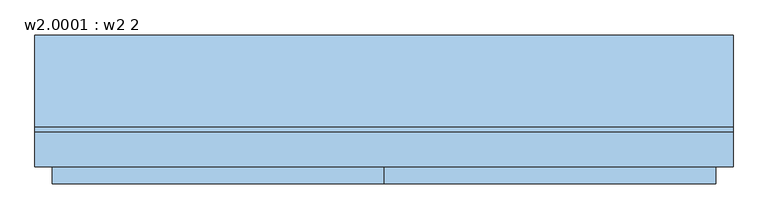
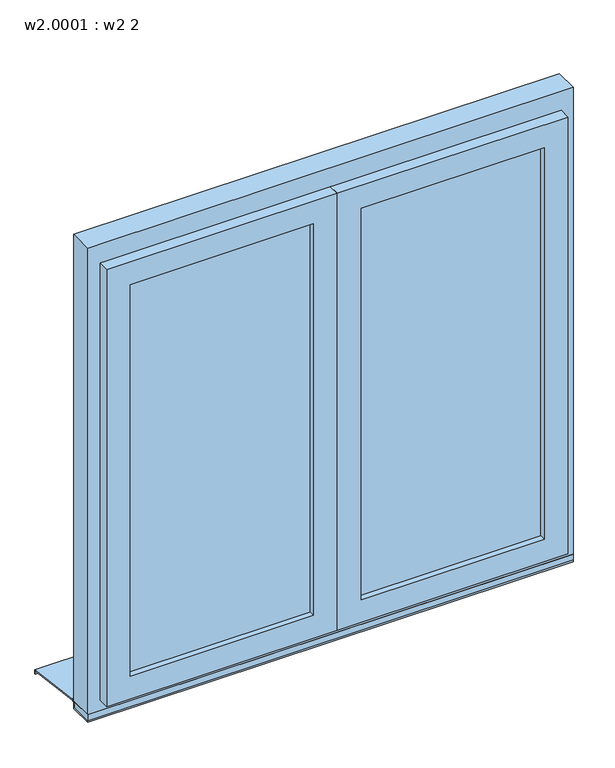
"""IFC4 building model written with IfcOpenShell, lengths in millimetres: window geometry, w2.0001 : w2 2."""

from ifc_helpers import new_model, si_unit, frame, origin, place, context, project, spatial, polyline, outline, extrude, faceted_brep, source, transform, mapped, element, save


def w2_0001_w2_2_f00e904a(model_context):
    return source(origin(), model_context, "Body", "SolidModel", [
        extrude(outline(polyline([(-72.8278457, 1020.0), (87.15, 1000.0), (87.15, 990.0), (85.15, 990.0), (85.15, 998.3604634), (-73.0259277, 1018.0), (-82.85, 1018.0), (-82.85, 1020.0), (-72.8278457, 1020.0)])), frame((-609.6, 0.0, 0.0), z_axis=(1.0, 0.0, 0.0), x_axis=(0.0, 1.0, 0.0)), (0.0, 0.0, 1.0), 1219.2),
        extrude(outline(polyline([(-609.6, -142.85), (-609.6, -87.15), (609.6, -87.15), (609.6, -142.85), (-609.6, -142.85)])), frame((0.0, 0.0, 1005.0), z_axis=(0.0, 0.0, 1.0), x_axis=(1.0, 0.0, 0.0)), (0.0, 0.0, 1.0), 15.0),
        extrude(outline(polyline([(60.0, -127.85), (519.6, -127.85), (519.6, -157.85), (60.0, -157.85), (60.0, -127.85)])), frame((0.0, 0.0, 1110.0), z_axis=(0.0, 0.0, 1.0), x_axis=(1.0, 0.0, 0.0)), (0.0, 0.0, 1.0), 1040.0),
        extrude(outline(polyline([(-519.6, -127.85), (-60.0, -127.85), (-60.0, -157.85), (-519.6, -157.85), (-519.6, -127.85)])), frame((0.0, 0.0, 1110.0), z_axis=(0.0, 0.0, 1.0), x_axis=(1.0, 0.0, 0.0)), (0.0, 0.0, 1.0), 1040.0),
        extrude(outline(polyline([(2260.0, -609.6), (1000.0, -609.6), (1000.0, 609.6), (2260.0, 609.6), (2260.0, -609.6)]), holes=[polyline([(2180.0, -549.6), (2180.0, 549.6), (1080.0, 549.6), (1080.0, -549.6), (2180.0, -549.6)])]), frame((0.0, -142.85, 0.0), z_axis=(0.0, 1.0, 0.0), x_axis=(0.0, 0.0, 1.0)), (0.0, 0.0, 1.0), 60.0),
        extrude(outline(polyline([(30.0, -142.85), (-30.0, -142.85), (-30.0, -82.85), (30.0, -82.85), (30.0, -142.85)])), frame((0.0, 0.0, 1080.0), z_axis=(0.0, 0.0, 1.0), x_axis=(1.0, 0.0, 0.0)), (0.0, 0.0, 1.0), 1100.0),
        faceted_brep([(30.0, -142.85, 1080.0), (30.0, -112.85, 1080.0), (549.6, -112.85, 1080.0), (549.6, -142.85, 1080.0), (549.6, -112.85, 2180.0), (549.6, -142.85, 2180.0), (30.0, -112.85, 2180.0), (519.6, -112.85, 2150.0), (60.0, -112.85, 2150.0), (60.0, -112.85, 1110.0), (519.6, -112.85, 1110.0), (579.6, -142.85, 1050.0), (0.0, -142.85, 1050.0), (0.0, -142.85, 2210.0), (579.6, -142.85, 2210.0), (30.0, -142.85, 2180.0), (0.0, -172.85, 1050.0), (579.6, -172.85, 1050.0), (579.6, -172.85, 2210.0), (0.0, -172.85, 2210.0), (519.6, -172.85, 1110.0), (60.0, -172.85, 1110.0), (60.0, -172.85, 2150.0), (519.6, -172.85, 2150.0)], [[[0, 1, 2, 3]], [[3, 2, 4, 5]], [[2, 1, 6, 4], [7, 8, 9, 10]], [[11, 12, 13, 14], [5, 15, 0, 3]], [[16, 12, 11, 17]], [[17, 11, 14, 18]], [[18, 19, 16, 17], [20, 21, 22, 23]], [[9, 21, 20, 10]], [[10, 20, 23, 7]], [[15, 6, 1, 0]], [[19, 13, 12, 16]], [[8, 22, 21, 9]], [[5, 4, 6, 15]], [[18, 14, 13, 19]], [[7, 23, 22, 8]]]),
        faceted_brep([(-549.6, -142.85, 1080.0), (-549.6, -112.85, 1080.0), (-30.0, -112.85, 1080.0), (-30.0, -142.85, 1080.0), (-30.0, -112.85, 2180.0), (-30.0, -142.85, 2180.0), (-549.6, -112.85, 2180.0), (-60.0, -112.85, 2150.0), (-519.6, -112.85, 2150.0), (-519.6, -112.85, 1110.0), (-60.0, -112.85, 1110.0), (0.0, -142.85, 1050.0), (-579.6, -142.85, 1050.0), (-579.6, -142.85, 2210.0), (0.0, -142.85, 2210.0), (-549.6, -142.85, 2180.0), (-579.6, -172.85, 1050.0), (0.0, -172.85, 1050.0), (0.0, -172.85, 2210.0), (-579.6, -172.85, 2210.0), (-60.0, -172.85, 1110.0), (-519.6, -172.85, 1110.0), (-519.6, -172.85, 2150.0), (-60.0, -172.85, 2150.0)], [[[0, 1, 2, 3]], [[3, 2, 4, 5]], [[2, 1, 6, 4], [7, 8, 9, 10]], [[11, 12, 13, 14], [5, 15, 0, 3]], [[16, 12, 11, 17]], [[17, 11, 14, 18]], [[18, 19, 16, 17], [20, 21, 22, 23]], [[9, 21, 20, 10]], [[10, 20, 23, 7]], [[15, 6, 1, 0]], [[19, 13, 12, 16]], [[8, 22, 21, 9]], [[5, 4, 6, 15]], [[18, 14, 13, 19]], [[7, 23, 22, 8]]]),
    ])


if __name__ == "__main__":
    model = new_model("IFC4")
    model_context = context("Model", 3, world=origin())
    ifc_project = project(units=[si_unit("LENGTHUNIT", "METRE", prefix="MILLI")], contexts=[model_context])
    site = spatial("IfcSite", under=ifc_project)
    building = spatial("IfcBuilding", under=site)
    placement = place(None, origin())
    w2_0001_w2_2_shape = w2_0001_w2_2_f00e904a(model_context)
    element("IfcWindow", 1, ObjectType="w2.0001 : w2 2", at=placement, inside=building, context=model_context, shape_type="MappedRepresentation", body=[
        mapped(w2_0001_w2_2_shape, transform((0.0, 0.0, 0.0), x_axis=(1.0, 0.0, 0.0), y_axis=(0.0, 1.0, 0.0), z_axis=(0.0, 0.0, 1.0))),
    ])
    save(model, "model.ifc")

# Revit data of these elements
# Type "w2.0001 : w2 2"
#   Type Mark = "20"
#   Operation = "DoublePanelVertical"
#   Keynote = "16.05.01"
#   Analytic Construction = "<None>"
#   Rough Width = 4' - 0"
#   Rough Height = 4' - 1.6063"
#   Rahmentiefe = 0' - 2.3622"
#   Rahmenhöhe unten = 0' - 3.14961"
#   Rahmehöhe oben = 0' - 3.14961"
#   Rahmenbreite = 0' - 2.3622"
#   Height = 4' - 1.6063"
#   Flügeltiefe = 0' - 2.3622"
#   Flügelbreite = 0' - 2.3622"
#   Einbautiefe (von außen) [instance default] = 0' - 5.51181"
#   Width = 4' - 0"
#   Kippflügel [instance default] = yes
#   Drehflügel im Grundriß darstellen [instance default] = no
#   Drehflügel [instance default] = yes
#   Define Thermal Properties by = 1
#   Rahmen [instance default] = none
#   Glas [instance default] = none
#   Flügel [instance default] = none
#   Fensterbank aussen [instance default] = none
#   Fensterbank innen [instance default] = none
#   Wall Closure = (empty or 0)
# Element 1 (IfcWindow, "w2.0001 : w2 2")
#   Materials on its faces: "Fenster - Kunststoff", "Fenster - Kunststoff weiss", "Glass", "Fenster - Holz"
# Materials
#   "Fenster - Kunststoff": colour RGB 249 249 249, transparency 0
#   "Fenster - Kunststoff weiss": colour RGB 249 249 249, transparency 0
#   "Glass": class "Glass", colour RGB 0 128 192, transparency 0.75, Description = "Soda Lime Glass", Cost = 0
#   "Fenster - Holz": colour RGB 216 135 75, transparency 0
